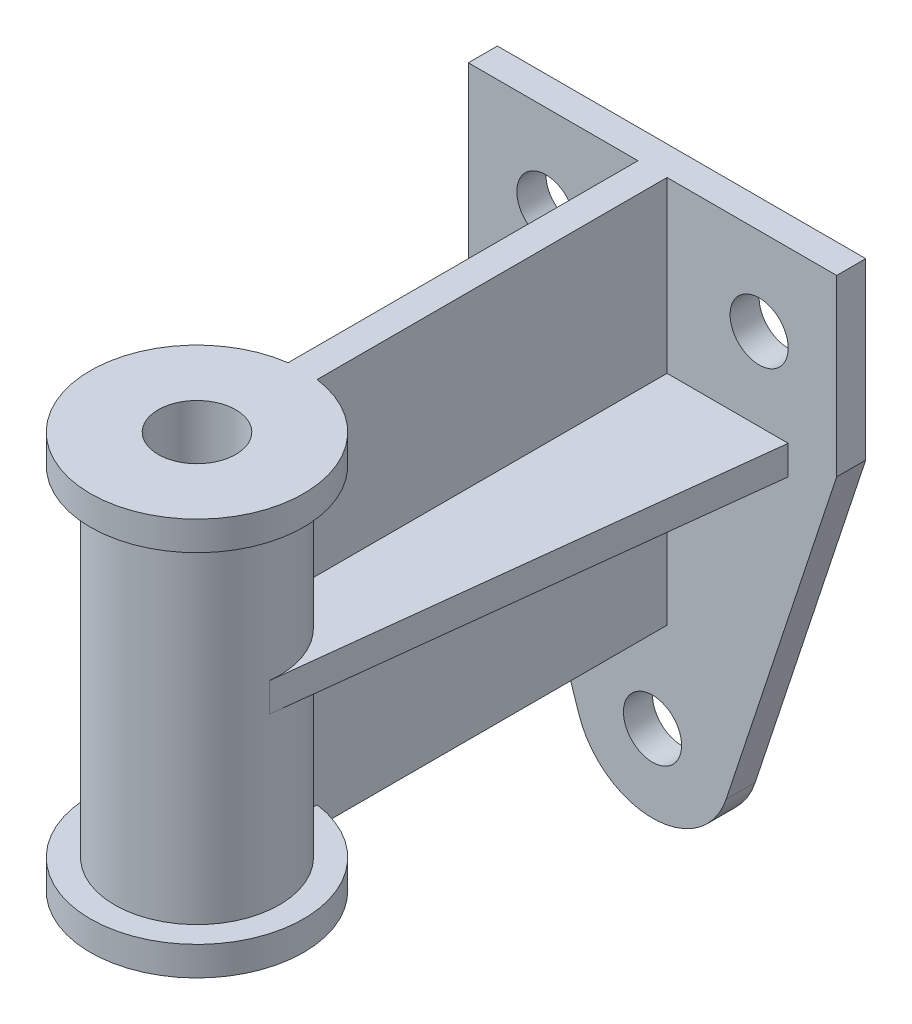
ISO-10303-21;
HEADER;
FILE_DESCRIPTION(('STEP AP214'),'2;1');
FILE_NAME('part.step','',(''),(''),'','','');
FILE_SCHEMA(('AUTOMOTIVE_DESIGN { 1 0 10303 214 1 1 1 1 }'));
ENDSEC;
DATA;
#1=APPLICATION_CONTEXT('core data for automotive mechanical design processes');
#2=APPLICATION_PROTOCOL_DEFINITION('international standard','automotive_design',2000,#1);
#3=PRODUCT_CONTEXT('',#1,'mechanical');
#4=PRODUCT('Part','Part','',(#3));
#5=PRODUCT_RELATED_PRODUCT_CATEGORY('part','',(#4));
#6=PRODUCT_DEFINITION_FORMATION('','',#4);
#7=PRODUCT_DEFINITION_CONTEXT('part definition',#1,'design');
#8=PRODUCT_DEFINITION('design','',#6,#7);
#9=PRODUCT_DEFINITION_SHAPE('','',#8);
#10=(LENGTH_UNIT() NAMED_UNIT(*) SI_UNIT(.MILLI.,.METRE.));
#11=(NAMED_UNIT(*) PLANE_ANGLE_UNIT() SI_UNIT($,.RADIAN.));
#12=(NAMED_UNIT(*) SI_UNIT($,.STERADIAN.) SOLID_ANGLE_UNIT());
#13=UNCERTAINTY_MEASURE_WITH_UNIT(LENGTH_MEASURE(1.E-05),#10,'distance_accuracy_value','');
#14=(GEOMETRIC_REPRESENTATION_CONTEXT(3) GLOBAL_UNCERTAINTY_ASSIGNED_CONTEXT((#13)) GLOBAL_UNIT_ASSIGNED_CONTEXT((#10,
#11,#12)) REPRESENTATION_CONTEXT('',''));
#15=CARTESIAN_POINT('',(0.,0.,0.));
#16=DIRECTION('',(0.,0.,1.));
#17=DIRECTION('',(1.,0.,0.));
#18=AXIS2_PLACEMENT_3D('',#15,#16,#17);
#19=CARTESIAN_POINT('',(0.,0.,6.));
#20=DIRECTION('',(0.,0.,1.));
#21=DIRECTION('',(1.,0.,0.));
#22=AXIS2_PLACEMENT_3D('',#19,#20,#21);
#23=PLANE('',#22);
#24=CARTESIAN_POINT('',(0.,0.,6.));
#25=DIRECTION('',(0.,0.,1.));
#26=DIRECTION('',(1.,0.,0.));
#27=AXIS2_PLACEMENT_3D('',#24,#25,#26);
#28=CIRCLE('',#27,6.);
#29=CARTESIAN_POINT('',(6.,0.,6.));
#30=VERTEX_POINT('',#29);
#31=EDGE_CURVE('E232',#30,#30,#28,.T.);
#32=ORIENTED_EDGE('',*,*,#31,.F.);
#33=EDGE_LOOP('',(#32));
#34=FACE_BOUND('',#33,.T.);
#35=CARTESIAN_POINT('',(-22.,82.,6.));
#36=DIRECTION('',(0.,0.,1.));
#37=DIRECTION('',(1.,0.,0.));
#38=AXIS2_PLACEMENT_3D('',#35,#36,#37);
#39=CIRCLE('',#38,6.);
#40=CARTESIAN_POINT('',(-16.,82.,6.));
#41=VERTEX_POINT('',#40);
#42=EDGE_CURVE('E240',#41,#41,#39,.T.);
#43=ORIENTED_EDGE('',*,*,#42,.F.);
#44=EDGE_LOOP('',(#43));
#45=FACE_BOUND('',#44,.T.);
#46=CARTESIAN_POINT('',(22.,82.,6.));
#47=DIRECTION('',(0.,0.,1.));
#48=DIRECTION('',(1.,0.,0.));
#49=AXIS2_PLACEMENT_3D('',#46,#47,#48);
#50=CIRCLE('',#49,6.);
#51=CARTESIAN_POINT('',(28.,82.,6.));
#52=VERTEX_POINT('',#51);
#53=EDGE_CURVE('E241',#52,#52,#50,.T.);
#54=ORIENTED_EDGE('',*,*,#53,.F.);
#55=EDGE_LOOP('',(#54));
#56=FACE_BOUND('',#55,.T.);
#57=DIRECTION('',(-1.,0.,0.));
#58=VECTOR('',#57,1.);
#59=CARTESIAN_POINT('',(-28.,59.,6.));
#60=LINE('',#59,#58);
#61=CARTESIAN_POINT('',(28.,59.,6.));
#62=VERTEX_POINT('',#61);
#63=CARTESIAN_POINT('',(2.99999999999999,59.,6.));
#64=VERTEX_POINT('',#63);
#65=EDGE_CURVE('E308',#62,#64,#60,.T.);
#66=ORIENTED_EDGE('',*,*,#65,.T.);
#67=DIRECTION('',(0.,1.,0.));
#68=VECTOR('',#67,1.);
#69=CARTESIAN_POINT('',(2.99999999999999,59.,6.));
#70=LINE('',#69,#68);
#71=CARTESIAN_POINT('',(3.,20.,6.));
#72=VERTEX_POINT('',#71);
#73=EDGE_CURVE('E61',#72,#64,#70,.T.);
#74=ORIENTED_EDGE('',*,*,#73,.F.);
#75=DIRECTION('',(1.,0.,0.));
#76=VECTOR('',#75,1.);
#77=CARTESIAN_POINT('',(-3.,20.,6.));
#78=LINE('',#77,#76);
#79=CARTESIAN_POINT('',(-3.,20.,6.));
#80=VERTEX_POINT('',#79);
#81=EDGE_CURVE('E59',#80,#72,#78,.T.);
#82=ORIENTED_EDGE('',*,*,#81,.F.);
#83=DIRECTION('',(0.,-1.,0.));
#84=VECTOR('',#83,1.);
#85=CARTESIAN_POINT('',(-3.00000000000001,59.,6.));
#86=LINE('',#85,#84);
#87=CARTESIAN_POINT('',(-3.00000000000001,59.,6.));
#88=VERTEX_POINT('',#87);
#89=EDGE_CURVE('E247',#88,#80,#86,.T.);
#90=ORIENTED_EDGE('',*,*,#89,.F.);
#91=CARTESIAN_POINT('',(-28.,59.,6.));
#92=VERTEX_POINT('',#91);
#93=EDGE_CURVE('E301',#88,#92,#60,.T.);
#94=ORIENTED_EDGE('',*,*,#93,.T.);
#95=DIRECTION('',(0.,1.,0.));
#96=VECTOR('',#95,1.);
#97=CARTESIAN_POINT('',(-28.,59.,6.));
#98=LINE('',#97,#96);
#99=CARTESIAN_POINT('',(-28.,65.,6.));
#100=VERTEX_POINT('',#99);
#101=EDGE_CURVE('E321',#92,#100,#98,.T.);
#102=ORIENTED_EDGE('',*,*,#101,.T.);
#103=DIRECTION('',(-1.,0.,0.));
#104=VECTOR('',#103,1.);
#105=CARTESIAN_POINT('',(-28.,65.,6.));
#106=LINE('',#105,#104);
#107=CARTESIAN_POINT('',(-3.00000000000001,65.,6.));
#108=VERTEX_POINT('',#107);
#109=EDGE_CURVE('E318',#108,#100,#106,.T.);
#110=ORIENTED_EDGE('',*,*,#109,.F.);
#111=DIRECTION('',(0.,-1.,0.));
#112=VECTOR('',#111,1.);
#113=CARTESIAN_POINT('',(-3.00000000000002,100.,6.));
#114=LINE('',#113,#112);
#115=CARTESIAN_POINT('',(-3.00000000000002,100.,6.));
#116=VERTEX_POINT('',#115);
#117=EDGE_CURVE('E246',#116,#108,#114,.T.);
#118=ORIENTED_EDGE('',*,*,#117,.F.);
#119=DIRECTION('',(-1.,0.,0.));
#120=VECTOR('',#119,1.);
#121=CARTESIAN_POINT('',(-38.,100.,6.));
#122=LINE('',#121,#120);
#123=CARTESIAN_POINT('',(-38.,100.,6.));
#124=VERTEX_POINT('',#123);
#125=EDGE_CURVE('E341',#116,#124,#122,.T.);
#126=ORIENTED_EDGE('',*,*,#125,.T.);
#127=DIRECTION('',(0.,-1.,0.));
#128=VECTOR('',#127,1.);
#129=CARTESIAN_POINT('',(-38.,100.,6.));
#130=LINE('',#129,#128);
#131=CARTESIAN_POINT('',(-38.,64.,6.));
#132=VERTEX_POINT('',#131);
#133=EDGE_CURVE('E334',#124,#132,#130,.T.);
#134=ORIENTED_EDGE('',*,*,#133,.T.);
#135=DIRECTION('',(0.313765855685688,-0.949500388523264,0.));
#136=VECTOR('',#135,1.);
#137=CARTESIAN_POINT('',(-38.,64.,6.));
#138=LINE('',#137,#136);
#139=CARTESIAN_POINT('',(-15.1920062163722,-5.020253690971,6.));
#140=VERTEX_POINT('',#139);
#141=EDGE_CURVE('E338',#132,#140,#138,.T.);
#142=ORIENTED_EDGE('',*,*,#141,.T.);
#143=CARTESIAN_POINT('',(0.,0.,6.));
#144=DIRECTION('',(0.,0.,1.));
#145=DIRECTION('',(1.,0.,0.));
#146=AXIS2_PLACEMENT_3D('',#143,#144,#145);
#147=CIRCLE('',#146,16.);
#148=CARTESIAN_POINT('',(15.1920062163722,-5.020253690971,6.));
#149=VERTEX_POINT('',#148);
#150=EDGE_CURVE('E337',#140,#149,#147,.T.);
#151=ORIENTED_EDGE('',*,*,#150,.T.);
#152=DIRECTION('',(0.313765855685688,0.949500388523264,0.));
#153=VECTOR('',#152,1.);
#154=CARTESIAN_POINT('',(38.,64.,6.));
#155=LINE('',#154,#153);
#156=CARTESIAN_POINT('',(38.,64.,6.));
#157=VERTEX_POINT('',#156);
#158=EDGE_CURVE('E342',#149,#157,#155,.T.);
#159=ORIENTED_EDGE('',*,*,#158,.T.);
#160=DIRECTION('',(0.,1.,0.));
#161=VECTOR('',#160,1.);
#162=CARTESIAN_POINT('',(38.,100.,6.));
#163=LINE('',#162,#161);
#164=CARTESIAN_POINT('',(38.,100.,6.));
#165=VERTEX_POINT('',#164);
#166=EDGE_CURVE('E343',#157,#165,#163,.T.);
#167=ORIENTED_EDGE('',*,*,#166,.T.);
#168=CARTESIAN_POINT('',(2.99999999999998,100.,6.));
#169=VERTEX_POINT('',#168);
#170=EDGE_CURVE('E347',#165,#169,#122,.T.);
#171=ORIENTED_EDGE('',*,*,#170,.T.);
#172=DIRECTION('',(0.,1.,0.));
#173=VECTOR('',#172,1.);
#174=CARTESIAN_POINT('',(2.99999999999998,100.,6.));
#175=LINE('',#174,#173);
#176=CARTESIAN_POINT('',(2.99999999999999,65.,6.));
#177=VERTEX_POINT('',#176);
#178=EDGE_CURVE('E250',#177,#169,#175,.T.);
#179=ORIENTED_EDGE('',*,*,#178,.F.);
#180=CARTESIAN_POINT('',(28.,65.,6.));
#181=VERTEX_POINT('',#180);
#182=EDGE_CURVE('E299',#181,#177,#106,.T.);
#183=ORIENTED_EDGE('',*,*,#182,.F.);
#184=DIRECTION('',(0.,1.,0.));
#185=VECTOR('',#184,1.);
#186=CARTESIAN_POINT('',(28.,59.,5.99999999999999));
#187=LINE('',#186,#185);
#188=EDGE_CURVE('E324',#62,#181,#187,.T.);
#189=ORIENTED_EDGE('',*,*,#188,.F.);
#190=EDGE_LOOP('',(#66,#74,#82,#90,#94,#102,#110,#118,#126,#134,#142,#151,#159,#167,#171,#179,
#183,#189));
#191=FACE_BOUND('',#190,.T.);
#192=ADVANCED_FACE('F43',(#34,#45,#56,#191),#23,.T.);
#193=CARTESIAN_POINT('',(0.,24.,100.));
#194=DIRECTION('',(0.,1.,0.));
#195=DIRECTION('',(-1.,0.,0.));
#196=AXIS2_PLACEMENT_3D('',#193,#194,#195);
#197=CYLINDRICAL_SURFACE('',#196,17.);
#198=DIRECTION('',(0.,1.,0.));
#199=VECTOR('',#198,1.);
#200=CARTESIAN_POINT('',(3.,24.,83.2667994693185));
#201=LINE('',#200,#199);
#202=CARTESIAN_POINT('',(3.,24.,83.2667994693185));
#203=VERTEX_POINT('',#202);
#204=CARTESIAN_POINT('',(2.99999999999999,59.,83.2667994693185));
#205=VERTEX_POINT('',#204);
#206=EDGE_CURVE('E432',#203,#205,#201,.T.);
#207=ORIENTED_EDGE('',*,*,#206,.T.);
#208=CARTESIAN_POINT('',(0.,59.,100.));
#209=DIRECTION('',(0.,-1.,0.));
#210=DIRECTION('',(0.,0.,1.));
#211=AXIS2_PLACEMENT_3D('',#208,#209,#210);
#212=CIRCLE('',#211,17.);
#213=CARTESIAN_POINT('',(16.887127655556,59.,101.955740152719));
#214=VERTEX_POINT('',#213);
#215=EDGE_CURVE('E297',#205,#214,#212,.T.);
#216=ORIENTED_EDGE('',*,*,#215,.T.);
#217=DIRECTION('',(0.,1.,0.));
#218=VECTOR('',#217,1.);
#219=CARTESIAN_POINT('',(16.887127655556,59.,101.955740152719));
#220=LINE('',#219,#218);
#221=CARTESIAN_POINT('',(16.887127655556,65.,101.955740152719));
#222=VERTEX_POINT('',#221);
#223=EDGE_CURVE('E327',#214,#222,#220,.T.);
#224=ORIENTED_EDGE('',*,*,#223,.T.);
#225=CARTESIAN_POINT('',(0.,65.,100.));
#226=DIRECTION('',(0.,-1.,0.));
#227=DIRECTION('',(0.,0.,1.));
#228=AXIS2_PLACEMENT_3D('',#225,#226,#227);
#229=CIRCLE('',#228,17.);
#230=CARTESIAN_POINT('',(2.99999999999999,65.,83.2667994693185));
#231=VERTEX_POINT('',#230);
#232=EDGE_CURVE('E313',#231,#222,#229,.T.);
#233=ORIENTED_EDGE('',*,*,#232,.F.);
#234=DIRECTION('',(0.,1.,0.));
#235=VECTOR('',#234,1.);
#236=CARTESIAN_POINT('',(2.99999999999999,24.,83.2667994693185));
#237=LINE('',#236,#235);
#238=CARTESIAN_POINT('',(3.00000000000001,94.,83.2667994693185));
#239=VERTEX_POINT('',#238);
#240=EDGE_CURVE('E229',#231,#239,#237,.T.);
#241=ORIENTED_EDGE('',*,*,#240,.T.);
#242=CARTESIAN_POINT('',(0.,94.,100.));
#243=DIRECTION('',(0.,-1.,0.));
#244=DIRECTION('',(1.,0.,0.));
#245=AXIS2_PLACEMENT_3D('',#242,#243,#244);
#246=CIRCLE('',#245,17.);
#247=CARTESIAN_POINT('',(-2.99999999999999,94.,83.2667994693185));
#248=VERTEX_POINT('',#247);
#249=EDGE_CURVE('E284',#239,#248,#246,.T.);
#250=ORIENTED_EDGE('',*,*,#249,.T.);
#251=DIRECTION('',(0.,1.,0.));
#252=VECTOR('',#251,1.);
#253=CARTESIAN_POINT('',(-3.,24.,83.2667994693185));
#254=LINE('',#253,#252);
#255=CARTESIAN_POINT('',(-3.00000000000001,65.,83.2667994693185));
#256=VERTEX_POINT('',#255);
#257=EDGE_CURVE('E261',#248,#256,#254,.F.);
#258=ORIENTED_EDGE('',*,*,#257,.T.);
#259=CARTESIAN_POINT('',(-16.887127655556,65.,101.955740152719));
#260=VERTEX_POINT('',#259);
#261=EDGE_CURVE('E315',#260,#256,#229,.T.);
#262=ORIENTED_EDGE('',*,*,#261,.F.);
#263=DIRECTION('',(0.,1.,0.));
#264=VECTOR('',#263,1.);
#265=CARTESIAN_POINT('',(-16.887127655556,59.,101.955740152719));
#266=LINE('',#265,#264);
#267=CARTESIAN_POINT('',(-16.887127655556,59.,101.955740152719));
#268=VERTEX_POINT('',#267);
#269=EDGE_CURVE('E306',#268,#260,#266,.T.);
#270=ORIENTED_EDGE('',*,*,#269,.F.);
#271=CARTESIAN_POINT('',(-3.00000000000001,59.,83.2667994693185));
#272=VERTEX_POINT('',#271);
#273=EDGE_CURVE('E209',#268,#272,#212,.T.);
#274=ORIENTED_EDGE('',*,*,#273,.T.);
#275=DIRECTION('',(0.,1.,0.));
#276=VECTOR('',#275,1.);
#277=CARTESIAN_POINT('',(-3.,24.,83.2667994693185));
#278=LINE('',#277,#276);
#279=CARTESIAN_POINT('',(-3.,24.,83.2667994693185));
#280=VERTEX_POINT('',#279);
#281=EDGE_CURVE('E210',#272,#280,#278,.F.);
#282=ORIENTED_EDGE('',*,*,#281,.T.);
#283=CARTESIAN_POINT('',(0.,24.,100.));
#284=DIRECTION('',(0.,-1.,0.));
#285=DIRECTION('',(1.,0.,0.));
#286=AXIS2_PLACEMENT_3D('',#283,#284,#285);
#287=CIRCLE('',#286,17.);
#288=EDGE_CURVE('E192',#203,#280,#287,.T.);
#289=ORIENTED_EDGE('',*,*,#288,.F.);
#290=EDGE_LOOP('',(#207,#216,#224,#233,#241,#250,#258,#262,#270,#274,#282,#289));
#291=FACE_BOUND('',#290,.T.);
#292=ADVANCED_FACE('F208',(#291),#197,.T.);
#293=CARTESIAN_POINT('',(0.,59.,100.));
#294=DIRECTION('',(0.,1.,0.));
#295=DIRECTION('',(0.,0.,1.));
#296=AXIS2_PLACEMENT_3D('',#293,#294,#295);
#297=PLANE('',#296);
#298=DIRECTION('',(0.,0.,-1.));
#299=VECTOR('',#298,1.);
#300=CARTESIAN_POINT('',(2.99999999999999,59.,122.002));
#301=LINE('',#300,#299);
#302=EDGE_CURVE('E421',#205,#64,#301,.T.);
#303=ORIENTED_EDGE('',*,*,#302,.T.);
#304=ORIENTED_EDGE('',*,*,#65,.F.);
#305=DIRECTION('',(0.115043538395224,0.,-0.993360450326822));
#306=VECTOR('',#305,1.);
#307=CARTESIAN_POINT('',(28.,59.,5.99999999999999));
#308=LINE('',#307,#306);
#309=EDGE_CURVE('E305',#214,#62,#308,.T.);
#310=ORIENTED_EDGE('',*,*,#309,.F.);
#311=ORIENTED_EDGE('',*,*,#215,.F.);
#312=EDGE_LOOP('',(#303,#304,#310,#311));
#313=FACE_BOUND('',#312,.T.);
#314=ADVANCED_FACE('F480',(#313),#297,.F.);
#315=DIRECTION('',(0.,0.,-1.));
#316=VECTOR('',#315,1.);
#317=CARTESIAN_POINT('',(-3.00000000000001,59.,122.002));
#318=LINE('',#317,#316);
#319=EDGE_CURVE('E426',#272,#88,#318,.T.);
#320=ORIENTED_EDGE('',*,*,#319,.F.);
#321=ORIENTED_EDGE('',*,*,#273,.F.);
#322=DIRECTION('',(0.115043538395223,0.,0.993360450326822));
#323=VECTOR('',#322,1.);
#324=CARTESIAN_POINT('',(-28.,59.,6.));
#325=LINE('',#324,#323);
#326=EDGE_CURVE('E298',#92,#268,#325,.T.);
#327=ORIENTED_EDGE('',*,*,#326,.F.);
#328=ORIENTED_EDGE('',*,*,#93,.F.);
#329=EDGE_LOOP('',(#320,#321,#327,#328));
#330=FACE_BOUND('',#329,.T.);
#331=ADVANCED_FACE('F441',(#330),#297,.F.);
#332=CARTESIAN_POINT('',(0.,18.,100.));
#333=DIRECTION('',(0.,1.,0.));
#334=DIRECTION('',(-1.,0.,0.));
#335=AXIS2_PLACEMENT_3D('',#332,#333,#334);
#336=CYLINDRICAL_SURFACE('',#335,22.);
#337=CARTESIAN_POINT('',(0.,18.,100.));
#338=DIRECTION('',(0.,-1.,0.));
#339=DIRECTION('',(1.,0.,0.));
#340=AXIS2_PLACEMENT_3D('',#337,#338,#339);
#341=CIRCLE('',#340,22.);
#342=CARTESIAN_POINT('',(22.,18.,100.));
#343=VERTEX_POINT('',#342);
#344=EDGE_CURVE('E201',#343,#343,#341,.T.);
#345=ORIENTED_EDGE('',*,*,#344,.F.);
#346=EDGE_LOOP('',(#345));
#347=FACE_BOUND('',#346,.T.);
#348=DIRECTION('',(0.,1.,0.));
#349=VECTOR('',#348,1.);
#350=CARTESIAN_POINT('',(3.,18.,78.2055052822966));
#351=LINE('',#350,#349);
#352=CARTESIAN_POINT('',(3.,20.,78.2055052822966));
#353=VERTEX_POINT('',#352);
#354=CARTESIAN_POINT('',(3.,24.,78.2055052822966));
#355=VERTEX_POINT('',#354);
#356=EDGE_CURVE('E228',#353,#355,#351,.T.);
#357=ORIENTED_EDGE('',*,*,#356,.T.);
#358=CARTESIAN_POINT('',(0.,24.,100.));
#359=DIRECTION('',(0.,-1.,0.));
#360=DIRECTION('',(1.,0.,0.));
#361=AXIS2_PLACEMENT_3D('',#358,#359,#360);
#362=CIRCLE('',#361,22.);
#363=CARTESIAN_POINT('',(-3.,24.,78.2055052822966));
#364=VERTEX_POINT('',#363);
#365=EDGE_CURVE('E281',#355,#364,#362,.T.);
#366=ORIENTED_EDGE('',*,*,#365,.T.);
#367=DIRECTION('',(0.,1.,0.));
#368=VECTOR('',#367,1.);
#369=CARTESIAN_POINT('',(-3.,18.,78.2055052822966));
#370=LINE('',#369,#368);
#371=CARTESIAN_POINT('',(-3.,20.,78.2055052822966));
#372=VERTEX_POINT('',#371);
#373=EDGE_CURVE('E217',#364,#372,#370,.F.);
#374=ORIENTED_EDGE('',*,*,#373,.T.);
#375=CARTESIAN_POINT('',(0.,20.,100.));
#376=DIRECTION('',(0.,1.,0.));
#377=DIRECTION('',(-1.,0.,0.));
#378=AXIS2_PLACEMENT_3D('',#375,#376,#377);
#379=CIRCLE('',#378,22.);
#380=EDGE_CURVE('E213',#372,#353,#379,.F.);
#381=ORIENTED_EDGE('',*,*,#380,.T.);
#382=EDGE_LOOP('',(#357,#366,#374,#381));
#383=FACE_BOUND('',#382,.T.);
#384=ADVANCED_FACE('F644',(#347,#383),#336,.T.);
#385=CARTESIAN_POINT('',(0.,24.,100.));
#386=DIRECTION('',(0.,-1.,0.));
#387=DIRECTION('',(1.,0.,0.));
#388=AXIS2_PLACEMENT_3D('',#385,#386,#387);
#389=PLANE('',#388);
#390=DIRECTION('',(0.,0.,1.));
#391=VECTOR('',#390,1.);
#392=CARTESIAN_POINT('',(3.,24.,122.002));
#393=LINE('',#392,#391);
#394=EDGE_CURVE('E200',#355,#203,#393,.T.);
#395=ORIENTED_EDGE('',*,*,#394,.T.);
#396=ORIENTED_EDGE('',*,*,#288,.T.);
#397=DIRECTION('',(0.,0.,-1.));
#398=VECTOR('',#397,1.);
#399=CARTESIAN_POINT('',(-3.,24.,122.002));
#400=LINE('',#399,#398);
#401=EDGE_CURVE('E198',#280,#364,#400,.T.);
#402=ORIENTED_EDGE('',*,*,#401,.T.);
#403=ORIENTED_EDGE('',*,*,#365,.F.);
#404=EDGE_LOOP('',(#395,#396,#402,#403));
#405=FACE_BOUND('',#404,.T.);
#406=ADVANCED_FACE('F193',(#405),#389,.F.);
#407=CARTESIAN_POINT('',(0.,65.,100.));
#408=DIRECTION('',(0.,1.,0.));
#409=DIRECTION('',(0.,0.,1.));
#410=AXIS2_PLACEMENT_3D('',#407,#408,#409);
#411=PLANE('',#410);
#412=ORIENTED_EDGE('',*,*,#182,.T.);
#413=DIRECTION('',(0.,0.,-1.));
#414=VECTOR('',#413,1.);
#415=CARTESIAN_POINT('',(2.99999999999999,65.,122.002));
#416=LINE('',#415,#414);
#417=EDGE_CURVE('E275',#231,#177,#416,.T.);
#418=ORIENTED_EDGE('',*,*,#417,.F.);
#419=ORIENTED_EDGE('',*,*,#232,.T.);
#420=DIRECTION('',(0.115043538395224,0.,-0.993360450326822));
#421=VECTOR('',#420,1.);
#422=CARTESIAN_POINT('',(28.,65.,5.99999999999999));
#423=LINE('',#422,#421);
#424=EDGE_CURVE('E312',#222,#181,#423,.T.);
#425=ORIENTED_EDGE('',*,*,#424,.T.);
#426=EDGE_LOOP('',(#412,#418,#419,#425));
#427=FACE_BOUND('',#426,.T.);
#428=ADVANCED_FACE('F409',(#427),#411,.T.);
#429=ORIENTED_EDGE('',*,*,#261,.T.);
#430=DIRECTION('',(0.,0.,-1.));
#431=VECTOR('',#430,1.);
#432=CARTESIAN_POINT('',(-3.00000000000001,65.,122.002));
#433=LINE('',#432,#431);
#434=EDGE_CURVE('E258',#256,#108,#433,.T.);
#435=ORIENTED_EDGE('',*,*,#434,.T.);
#436=ORIENTED_EDGE('',*,*,#109,.T.);
#437=DIRECTION('',(0.115043538395223,0.,0.993360450326822));
#438=VECTOR('',#437,1.);
#439=CARTESIAN_POINT('',(-28.,65.,6.));
#440=LINE('',#439,#438);
#441=EDGE_CURVE('E288',#100,#260,#440,.T.);
#442=ORIENTED_EDGE('',*,*,#441,.T.);
#443=EDGE_LOOP('',(#429,#435,#436,#442));
#444=FACE_BOUND('',#443,.T.);
#445=ADVANCED_FACE('F452',(#444),#411,.T.);
#446=CARTESIAN_POINT('',(0.,94.,100.));
#447=DIRECTION('',(0.,1.,0.));
#448=DIRECTION('',(-1.,0.,0.));
#449=AXIS2_PLACEMENT_3D('',#446,#447,#448);
#450=CYLINDRICAL_SURFACE('',#449,22.);
#451=CARTESIAN_POINT('',(0.,94.,100.));
#452=DIRECTION('',(0.,1.,0.));
#453=DIRECTION('',(-1.,0.,0.));
#454=AXIS2_PLACEMENT_3D('',#451,#452,#453);
#455=CIRCLE('',#454,22.);
#456=CARTESIAN_POINT('',(-3.00000000000002,94.,78.2055052822966));
#457=VERTEX_POINT('',#456);
#458=CARTESIAN_POINT('',(2.99999999999998,94.,78.2055052822966));
#459=VERTEX_POINT('',#458);
#460=EDGE_CURVE('E289',#457,#459,#455,.T.);
#461=ORIENTED_EDGE('',*,*,#460,.T.);
#462=DIRECTION('',(0.,1.,0.));
#463=VECTOR('',#462,1.);
#464=CARTESIAN_POINT('',(2.99999999999998,94.,78.2055052822966));
#465=LINE('',#464,#463);
#466=CARTESIAN_POINT('',(2.99999999999998,100.,78.2055052822966));
#467=VERTEX_POINT('',#466);
#468=EDGE_CURVE('E255',#467,#459,#465,.F.);
#469=ORIENTED_EDGE('',*,*,#468,.F.);
#470=CARTESIAN_POINT('',(0.,100.,100.));
#471=DIRECTION('',(0.,1.,0.));
#472=DIRECTION('',(-1.,0.,0.));
#473=AXIS2_PLACEMENT_3D('',#470,#471,#472);
#474=CIRCLE('',#473,22.);
#475=CARTESIAN_POINT('',(-3.00000000000002,100.,78.2055052822966));
#476=VERTEX_POINT('',#475);
#477=EDGE_CURVE('E205',#476,#467,#474,.T.);
#478=ORIENTED_EDGE('',*,*,#477,.F.);
#479=DIRECTION('',(0.,1.,0.));
#480=VECTOR('',#479,1.);
#481=CARTESIAN_POINT('',(-3.00000000000002,94.,78.2055052822966));
#482=LINE('',#481,#480);
#483=EDGE_CURVE('E260',#457,#476,#482,.T.);
#484=ORIENTED_EDGE('',*,*,#483,.F.);
#485=EDGE_LOOP('',(#461,#469,#478,#484));
#486=FACE_BOUND('',#485,.T.);
#487=ADVANCED_FACE('F458',(#486),#450,.T.);
#488=CARTESIAN_POINT('',(0.,94.,100.));
#489=DIRECTION('',(0.,1.,0.));
#490=DIRECTION('',(-1.,0.,0.));
#491=AXIS2_PLACEMENT_3D('',#488,#489,#490);
#492=PLANE('',#491);
#493=DIRECTION('',(0.,0.,-1.));
#494=VECTOR('',#493,1.);
#495=CARTESIAN_POINT('',(2.99999999999998,94.,122.002));
#496=LINE('',#495,#494);
#497=EDGE_CURVE('E262',#239,#459,#496,.T.);
#498=ORIENTED_EDGE('',*,*,#497,.T.);
#499=ORIENTED_EDGE('',*,*,#460,.F.);
#500=DIRECTION('',(0.,0.,1.));
#501=VECTOR('',#500,1.);
#502=CARTESIAN_POINT('',(-3.00000000000002,94.,122.002));
#503=LINE('',#502,#501);
#504=EDGE_CURVE('E257',#457,#248,#503,.T.);
#505=ORIENTED_EDGE('',*,*,#504,.T.);
#506=ORIENTED_EDGE('',*,*,#249,.F.);
#507=EDGE_LOOP('',(#498,#499,#505,#506));
#508=FACE_BOUND('',#507,.T.);
#509=ADVANCED_FACE('F457',(#508),#492,.F.);
#510=CARTESIAN_POINT('',(-38.,100.,6.));
#511=DIRECTION('',(1.,0.,0.));
#512=DIRECTION('',(0.,1.,0.));
#513=AXIS2_PLACEMENT_3D('',#510,#511,#512);
#514=PLANE('',#513);
#515=DIRECTION('',(0.,-1.,0.));
#516=VECTOR('',#515,1.);
#517=CARTESIAN_POINT('',(-38.,100.,0.));
#518=LINE('',#517,#516);
#519=CARTESIAN_POINT('',(-38.,100.,0.));
#520=VERTEX_POINT('',#519);
#521=CARTESIAN_POINT('',(-38.,64.,0.));
#522=VERTEX_POINT('',#521);
#523=EDGE_CURVE('E322',#520,#522,#518,.T.);
#524=ORIENTED_EDGE('',*,*,#523,.T.);
#525=DIRECTION('',(0.,0.,-1.));
#526=VECTOR('',#525,1.);
#527=CARTESIAN_POINT('',(-38.,64.,6.));
#528=LINE('',#527,#526);
#529=EDGE_CURVE('E11',#132,#522,#528,.T.);
#530=ORIENTED_EDGE('',*,*,#529,.F.);
#531=ORIENTED_EDGE('',*,*,#133,.F.);
#532=DIRECTION('',(0.,0.,-1.));
#533=VECTOR('',#532,1.);
#534=CARTESIAN_POINT('',(-38.,100.,6.));
#535=LINE('',#534,#533);
#536=EDGE_CURVE('E349',#124,#520,#535,.T.);
#537=ORIENTED_EDGE('',*,*,#536,.T.);
#538=EDGE_LOOP('',(#524,#530,#531,#537));
#539=FACE_BOUND('',#538,.T.);
#540=ADVANCED_FACE('F44',(#539),#514,.F.);
#541=CARTESIAN_POINT('',(-38.,64.,6.));
#542=DIRECTION('',(0.949500388523263,0.313765855685687,0.));
#543=DIRECTION('',(-0.313765855685688,0.949500388523264,0.));
#544=AXIS2_PLACEMENT_3D('',#541,#542,#543);
#545=PLANE('',#544);
#546=DIRECTION('',(0.313765855685688,-0.949500388523264,0.));
#547=VECTOR('',#546,1.);
#548=CARTESIAN_POINT('',(-38.,64.,0.));
#549=LINE('',#548,#547);
#550=CARTESIAN_POINT('',(-15.1920062163722,-5.020253690971,0.));
#551=VERTEX_POINT('',#550);
#552=EDGE_CURVE('E355',#522,#551,#549,.T.);
#553=ORIENTED_EDGE('',*,*,#552,.T.);
#554=DIRECTION('',(0.,0.,-1.));
#555=VECTOR('',#554,1.);
#556=CARTESIAN_POINT('',(-15.1920062163722,-5.020253690971,6.));
#557=LINE('',#556,#555);
#558=EDGE_CURVE('E51',#140,#551,#557,.T.);
#559=ORIENTED_EDGE('',*,*,#558,.F.);
#560=ORIENTED_EDGE('',*,*,#141,.F.);
#561=ORIENTED_EDGE('',*,*,#529,.T.);
#562=EDGE_LOOP('',(#553,#559,#560,#561));
#563=FACE_BOUND('',#562,.T.);
#564=ADVANCED_FACE('F400',(#563),#545,.F.);
#565=CARTESIAN_POINT('',(0.,0.,6.));
#566=DIRECTION('',(0.,0.,-1.));
#567=DIRECTION('',(-1.,0.,0.));
#568=AXIS2_PLACEMENT_3D('',#565,#566,#567);
#569=CYLINDRICAL_SURFACE('',#568,16.);
#570=CARTESIAN_POINT('',(0.,0.,0.));
#571=DIRECTION('',(0.,0.,1.));
#572=DIRECTION('',(1.,0.,0.));
#573=AXIS2_PLACEMENT_3D('',#570,#571,#572);
#574=CIRCLE('',#573,16.);
#575=CARTESIAN_POINT('',(15.1920062163722,-5.020253690971,0.));
#576=VERTEX_POINT('',#575);
#577=EDGE_CURVE('E352',#551,#576,#574,.T.);
#578=ORIENTED_EDGE('',*,*,#577,.T.);
#579=DIRECTION('',(0.,0.,-1.));
#580=VECTOR('',#579,1.);
#581=CARTESIAN_POINT('',(15.1920062163722,-5.020253690971,6.));
#582=LINE('',#581,#580);
#583=EDGE_CURVE('E369',#149,#576,#582,.T.);
#584=ORIENTED_EDGE('',*,*,#583,.F.);
#585=ORIENTED_EDGE('',*,*,#150,.F.);
#586=ORIENTED_EDGE('',*,*,#558,.T.);
#587=EDGE_LOOP('',(#578,#584,#585,#586));
#588=FACE_BOUND('',#587,.T.);
#589=ADVANCED_FACE('F376',(#588),#569,.T.);
#590=CARTESIAN_POINT('',(38.,64.,6.));
#591=DIRECTION('',(-0.949500388523263,0.313765855685687,0.));
#592=DIRECTION('',(-0.313765855685688,-0.949500388523264,0.));
#593=AXIS2_PLACEMENT_3D('',#590,#591,#592);
#594=PLANE('',#593);
#595=DIRECTION('',(0.313765855685688,0.949500388523264,0.));
#596=VECTOR('',#595,1.);
#597=CARTESIAN_POINT('',(38.,64.,0.));
#598=LINE('',#597,#596);
#599=CARTESIAN_POINT('',(38.,64.,0.));
#600=VERTEX_POINT('',#599);
#601=EDGE_CURVE('E357',#576,#600,#598,.T.);
#602=ORIENTED_EDGE('',*,*,#601,.T.);
#603=DIRECTION('',(0.,0.,-1.));
#604=VECTOR('',#603,1.);
#605=CARTESIAN_POINT('',(38.,64.,6.));
#606=LINE('',#605,#604);
#607=EDGE_CURVE('E368',#157,#600,#606,.T.);
#608=ORIENTED_EDGE('',*,*,#607,.F.);
#609=ORIENTED_EDGE('',*,*,#158,.F.);
#610=ORIENTED_EDGE('',*,*,#583,.T.);
#611=EDGE_LOOP('',(#602,#608,#609,#610));
#612=FACE_BOUND('',#611,.T.);
#613=ADVANCED_FACE('F390',(#612),#594,.F.);
#614=CARTESIAN_POINT('',(38.,100.,6.));
#615=DIRECTION('',(-1.,0.,0.));
#616=DIRECTION('',(0.,-1.,0.));
#617=AXIS2_PLACEMENT_3D('',#614,#615,#616);
#618=PLANE('',#617);
#619=DIRECTION('',(0.,1.,0.));
#620=VECTOR('',#619,1.);
#621=CARTESIAN_POINT('',(38.,100.,0.));
#622=LINE('',#621,#620);
#623=CARTESIAN_POINT('',(38.,100.,0.));
#624=VERTEX_POINT('',#623);
#625=EDGE_CURVE('E358',#600,#624,#622,.T.);
#626=ORIENTED_EDGE('',*,*,#625,.T.);
#627=DIRECTION('',(0.,0.,-1.));
#628=VECTOR('',#627,1.);
#629=CARTESIAN_POINT('',(38.,100.,6.));
#630=LINE('',#629,#628);
#631=EDGE_CURVE('E361',#165,#624,#630,.T.);
#632=ORIENTED_EDGE('',*,*,#631,.F.);
#633=ORIENTED_EDGE('',*,*,#166,.F.);
#634=ORIENTED_EDGE('',*,*,#607,.T.);
#635=EDGE_LOOP('',(#626,#632,#633,#634));
#636=FACE_BOUND('',#635,.T.);
#637=ADVANCED_FACE('F393',(#636),#618,.F.);
#638=CARTESIAN_POINT('',(-38.,100.,6.));
#639=DIRECTION('',(0.,-1.,0.));
#640=DIRECTION('',(1.,0.,0.));
#641=AXIS2_PLACEMENT_3D('',#638,#639,#640);
#642=PLANE('',#641);
#643=DIRECTION('',(-1.,0.,0.));
#644=VECTOR('',#643,1.);
#645=CARTESIAN_POINT('',(-38.,100.,0.));
#646=LINE('',#645,#644);
#647=EDGE_CURVE('E340',#624,#520,#646,.T.);
#648=ORIENTED_EDGE('',*,*,#647,.T.);
#649=ORIENTED_EDGE('',*,*,#536,.F.);
#650=ORIENTED_EDGE('',*,*,#125,.F.);
#651=DIRECTION('',(0.,0.,-1.));
#652=VECTOR('',#651,1.);
#653=CARTESIAN_POINT('',(-3.00000000000002,100.,122.002));
#654=LINE('',#653,#652);
#655=EDGE_CURVE('E253',#476,#116,#654,.T.);
#656=ORIENTED_EDGE('',*,*,#655,.F.);
#657=ORIENTED_EDGE('',*,*,#477,.T.);
#658=DIRECTION('',(0.,0.,-1.));
#659=VECTOR('',#658,1.);
#660=CARTESIAN_POINT('',(2.99999999999998,100.,122.002));
#661=LINE('',#660,#659);
#662=EDGE_CURVE('E269',#467,#169,#661,.T.);
#663=ORIENTED_EDGE('',*,*,#662,.T.);
#664=ORIENTED_EDGE('',*,*,#170,.F.);
#665=ORIENTED_EDGE('',*,*,#631,.T.);
#666=EDGE_LOOP('',(#648,#649,#650,#656,#657,#663,#664,#665));
#667=FACE_BOUND('',#666,.T.);
#668=CARTESIAN_POINT('',(0.,100.,100.));
#669=DIRECTION('',(0.,1.,0.));
#670=DIRECTION('',(-1.,0.,0.));
#671=AXIS2_PLACEMENT_3D('',#668,#669,#670);
#672=CIRCLE('',#671,8.);
#673=CARTESIAN_POINT('',(-8.00000000000002,100.,100.));
#674=VERTEX_POINT('',#673);
#675=EDGE_CURVE('E251',#674,#674,#672,.T.);
#676=ORIENTED_EDGE('',*,*,#675,.F.);
#677=EDGE_LOOP('',(#676));
#678=FACE_BOUND('',#677,.T.);
#679=ADVANCED_FACE('F402',(#667,#678),#642,.F.);
#680=CARTESIAN_POINT('',(0.,0.,0.));
#681=DIRECTION('',(0.,0.,1.));
#682=DIRECTION('',(1.,0.,0.));
#683=AXIS2_PLACEMENT_3D('',#680,#681,#682);
#684=PLANE('',#683);
#685=CARTESIAN_POINT('',(0.,0.,0.));
#686=DIRECTION('',(0.,0.,1.));
#687=DIRECTION('',(1.,0.,0.));
#688=AXIS2_PLACEMENT_3D('',#685,#686,#687);
#689=CIRCLE('',#688,6.);
#690=CARTESIAN_POINT('',(6.,0.,0.));
#691=VERTEX_POINT('',#690);
#692=EDGE_CURVE('E230',#691,#691,#689,.T.);
#693=ORIENTED_EDGE('',*,*,#692,.T.);
#694=EDGE_LOOP('',(#693));
#695=FACE_BOUND('',#694,.T.);
#696=CARTESIAN_POINT('',(-22.,82.,0.));
#697=DIRECTION('',(0.,0.,1.));
#698=DIRECTION('',(1.,0.,0.));
#699=AXIS2_PLACEMENT_3D('',#696,#697,#698);
#700=CIRCLE('',#699,6.);
#701=CARTESIAN_POINT('',(-16.,82.,0.));
#702=VERTEX_POINT('',#701);
#703=EDGE_CURVE('E234',#702,#702,#700,.T.);
#704=ORIENTED_EDGE('',*,*,#703,.T.);
#705=EDGE_LOOP('',(#704));
#706=FACE_BOUND('',#705,.T.);
#707=CARTESIAN_POINT('',(22.,82.,0.));
#708=DIRECTION('',(0.,0.,1.));
#709=DIRECTION('',(1.,0.,0.));
#710=AXIS2_PLACEMENT_3D('',#707,#708,#709);
#711=CIRCLE('',#710,6.);
#712=CARTESIAN_POINT('',(28.,82.,0.));
#713=VERTEX_POINT('',#712);
#714=EDGE_CURVE('E238',#713,#713,#711,.T.);
#715=ORIENTED_EDGE('',*,*,#714,.T.);
#716=EDGE_LOOP('',(#715));
#717=FACE_BOUND('',#716,.T.);
#718=ORIENTED_EDGE('',*,*,#523,.F.);
#719=ORIENTED_EDGE('',*,*,#647,.F.);
#720=ORIENTED_EDGE('',*,*,#625,.F.);
#721=ORIENTED_EDGE('',*,*,#601,.F.);
#722=ORIENTED_EDGE('',*,*,#577,.F.);
#723=ORIENTED_EDGE('',*,*,#552,.F.);
#724=EDGE_LOOP('',(#718,#719,#720,#721,#722,#723));
#725=FACE_BOUND('',#724,.T.);
#726=ADVANCED_FACE('F385',(#695,#706,#717,#725),#684,.F.);
#727=CARTESIAN_POINT('',(-28.,59.,6.));
#728=DIRECTION('',(-0.993360450326822,0.,0.115043538395223));
#729=DIRECTION('',(0.115043538395223,0.,0.993360450326822));
#730=AXIS2_PLACEMENT_3D('',#727,#728,#729);
#731=PLANE('',#730);
#732=ORIENTED_EDGE('',*,*,#441,.F.);
#733=ORIENTED_EDGE('',*,*,#101,.F.);
#734=ORIENTED_EDGE('',*,*,#326,.T.);
#735=ORIENTED_EDGE('',*,*,#269,.T.);
#736=EDGE_LOOP('',(#732,#733,#734,#735));
#737=FACE_BOUND('',#736,.T.);
#738=ADVANCED_FACE('F450',(#737),#731,.T.);
#739=CARTESIAN_POINT('',(28.,59.,5.99999999999999));
#740=DIRECTION('',(0.993360450326822,0.,0.115043538395224));
#741=DIRECTION('',(0.115043538395224,0.,-0.993360450326822));
#742=AXIS2_PLACEMENT_3D('',#739,#740,#741);
#743=PLANE('',#742);
#744=ORIENTED_EDGE('',*,*,#424,.F.);
#745=ORIENTED_EDGE('',*,*,#223,.F.);
#746=ORIENTED_EDGE('',*,*,#309,.T.);
#747=ORIENTED_EDGE('',*,*,#188,.T.);
#748=EDGE_LOOP('',(#744,#745,#746,#747));
#749=FACE_BOUND('',#748,.T.);
#750=ADVANCED_FACE('F411',(#749),#743,.T.);
#751=CARTESIAN_POINT('',(0.,18.,100.));
#752=DIRECTION('',(0.,-1.,0.));
#753=DIRECTION('',(1.,0.,0.));
#754=AXIS2_PLACEMENT_3D('',#751,#752,#753);
#755=PLANE('',#754);
#756=CARTESIAN_POINT('',(0.,18.,100.));
#757=DIRECTION('',(0.,-1.,0.));
#758=DIRECTION('',(1.,0.,0.));
#759=AXIS2_PLACEMENT_3D('',#756,#757,#758);
#760=CIRCLE('',#759,8.);
#761=CARTESIAN_POINT('',(-8.00000000000003,18.,100.));
#762=VERTEX_POINT('',#761);
#763=EDGE_CURVE('E278',#762,#762,#760,.T.);
#764=ORIENTED_EDGE('',*,*,#763,.F.);
#765=EDGE_LOOP('',(#764));
#766=FACE_BOUND('',#765,.T.);
#767=ORIENTED_EDGE('',*,*,#344,.T.);
#768=EDGE_LOOP('',(#767));
#769=FACE_BOUND('',#768,.T.);
#770=ADVANCED_FACE('F550',(#766,#769),#755,.T.);
#771=CARTESIAN_POINT('',(0.,-16.,100.));
#772=DIRECTION('',(0.,1.,0.));
#773=DIRECTION('',(-1.,0.,0.));
#774=AXIS2_PLACEMENT_3D('',#771,#772,#773);
#775=CYLINDRICAL_SURFACE('',#774,8.);
#776=CARTESIAN_POINT('',(-8.00000000000003,18.,100.));
#777=CARTESIAN_POINT('',(-8.00000000000003,18.8541666666667,100.));
#778=CARTESIAN_POINT('',(-8.00000000000003,19.7083333333333,100.));
#779=CARTESIAN_POINT('',(-8.00000000000003,21.4166666666667,100.));
#780=CARTESIAN_POINT('',(-8.00000000000003,22.2708333333333,100.));
#781=CARTESIAN_POINT('',(-8.00000000000003,23.9791666666667,100.));
#782=CARTESIAN_POINT('',(-8.00000000000003,24.8333333333333,100.));
#783=CARTESIAN_POINT('',(-8.00000000000003,26.5416666666666,100.));
#784=CARTESIAN_POINT('',(-8.00000000000003,27.3958333333333,100.));
#785=CARTESIAN_POINT('',(-8.00000000000003,29.1041666666667,100.));
#786=CARTESIAN_POINT('',(-8.00000000000003,29.9583333333333,100.));
#787=CARTESIAN_POINT('',(-8.00000000000003,31.6666666666667,100.));
#788=CARTESIAN_POINT('',(-8.00000000000003,32.5208333333333,100.));
#789=CARTESIAN_POINT('',(-8.00000000000003,34.2291666666667,100.));
#790=CARTESIAN_POINT('',(-8.00000000000003,35.0833333333333,100.));
#791=CARTESIAN_POINT('',(-8.00000000000003,36.7916666666667,100.));
#792=CARTESIAN_POINT('',(-8.00000000000003,37.6458333333333,100.));
#793=CARTESIAN_POINT('',(-8.00000000000003,39.3541666666667,100.));
#794=CARTESIAN_POINT('',(-8.00000000000003,40.2083333333333,100.));
#795=CARTESIAN_POINT('',(-8.00000000000003,41.9166666666667,100.));
#796=CARTESIAN_POINT('',(-8.00000000000003,42.7708333333333,100.));
#797=CARTESIAN_POINT('',(-8.00000000000003,44.4791666666667,100.));
#798=CARTESIAN_POINT('',(-8.00000000000003,45.3333333333333,100.));
#799=CARTESIAN_POINT('',(-8.00000000000003,47.0416666666667,100.));
#800=CARTESIAN_POINT('',(-8.00000000000003,47.8958333333333,100.));
#801=CARTESIAN_POINT('',(-8.00000000000003,49.6041666666666,100.));
#802=CARTESIAN_POINT('',(-8.00000000000003,50.4583333333333,100.));
#803=CARTESIAN_POINT('',(-8.00000000000003,52.1666666666666,100.));
#804=CARTESIAN_POINT('',(-8.00000000000003,53.0208333333333,100.));
#805=CARTESIAN_POINT('',(-8.00000000000003,54.7291666666667,100.));
#806=CARTESIAN_POINT('',(-8.00000000000003,55.5833333333333,100.));
#807=CARTESIAN_POINT('',(-8.00000000000003,57.2916666666667,100.));
#808=CARTESIAN_POINT('',(-8.00000000000003,58.1458333333333,100.));
#809=CARTESIAN_POINT('',(-8.00000000000003,59.8541666666666,100.));
#810=CARTESIAN_POINT('',(-8.00000000000003,60.7083333333333,100.));
#811=CARTESIAN_POINT('',(-8.00000000000003,62.4166666666667,100.));
#812=CARTESIAN_POINT('',(-8.00000000000003,63.2708333333333,100.));
#813=CARTESIAN_POINT('',(-8.00000000000003,64.9791666666667,100.));
#814=CARTESIAN_POINT('',(-8.00000000000002,65.8333333333333,100.));
#815=CARTESIAN_POINT('',(-8.00000000000002,67.5416666666667,100.));
#816=CARTESIAN_POINT('',(-8.00000000000002,68.3958333333333,100.));
#817=CARTESIAN_POINT('',(-8.00000000000002,70.1041666666667,100.));
#818=CARTESIAN_POINT('',(-8.00000000000002,70.9583333333333,100.));
#819=CARTESIAN_POINT('',(-8.00000000000002,72.6666666666667,100.));
#820=CARTESIAN_POINT('',(-8.00000000000002,73.5208333333333,100.));
#821=CARTESIAN_POINT('',(-8.00000000000002,75.2291666666667,100.));
#822=CARTESIAN_POINT('',(-8.00000000000002,76.0833333333333,100.));
#823=CARTESIAN_POINT('',(-8.00000000000002,77.7916666666666,100.));
#824=CARTESIAN_POINT('',(-8.00000000000002,78.6458333333333,100.));
#825=CARTESIAN_POINT('',(-8.00000000000002,80.3541666666667,100.));
#826=CARTESIAN_POINT('',(-8.00000000000002,81.2083333333333,100.));
#827=CARTESIAN_POINT('',(-8.00000000000002,82.9166666666667,100.));
#828=CARTESIAN_POINT('',(-8.00000000000002,83.7708333333333,100.));
#829=CARTESIAN_POINT('',(-8.00000000000002,85.4791666666667,100.));
#830=CARTESIAN_POINT('',(-8.00000000000002,86.3333333333333,100.));
#831=CARTESIAN_POINT('',(-8.00000000000002,88.0416666666667,100.));
#832=CARTESIAN_POINT('',(-8.00000000000002,88.8958333333333,100.));
#833=CARTESIAN_POINT('',(-8.00000000000002,90.6041666666667,100.));
#834=CARTESIAN_POINT('',(-8.00000000000002,91.4583333333333,100.));
#835=CARTESIAN_POINT('',(-8.00000000000002,93.1666666666667,100.));
#836=CARTESIAN_POINT('',(-8.00000000000002,94.0208333333333,100.));
#837=CARTESIAN_POINT('',(-8.00000000000002,95.7291666666667,100.));
#838=CARTESIAN_POINT('',(-8.00000000000002,96.5833333333333,100.));
#839=CARTESIAN_POINT('',(-8.00000000000002,98.2916666666667,100.));
#840=CARTESIAN_POINT('',(-8.00000000000002,99.1458333333333,100.));
#841=CARTESIAN_POINT('',(-8.00000000000002,100.,100.));
#842=B_SPLINE_CURVE_WITH_KNOTS('',3,(#776,#777,#778,#779,#780,#781,#782,#783,#784,#785,#786,
#787,#788,#789,#790,#791,#792,#793,#794,#795,#796,#797,#798,#799,#800,#801,#802,#803,#804,#805,
#806,#807,#808,#809,#810,#811,#812,#813,#814,#815,#816,#817,#818,#819,#820,#821,#822,#823,#824,
#825,#826,#827,#828,#829,#830,#831,#832,#833,#834,#835,#836,#837,#838,#839,#840,#841),
.UNSPECIFIED.,.F.,.F.,(4,2,2,2,2,2,2,2,2,2,2,2,2,2,2,2,2,2,2,2,2,2,2,2,2,2,2,2,2,2,2,2,4),(0.,
2.5625,5.125,7.6875,10.25,12.8125,15.375,17.9375,20.5,23.0625,25.625,28.1875,30.75,33.3125,
35.875,38.4375,41.,43.5625,46.125,48.6875,51.25,53.8125,56.375,58.9375,61.5,64.0625,66.625,
69.1875,71.75,74.3125,76.875,79.4375,82.),.UNSPECIFIED.);
#843=EDGE_CURVE('BSEAM555',#762,#674,#842,.T.);
#844=ORIENTED_EDGE('',*,*,#763,.T.);
#845=ORIENTED_EDGE('',*,*,#675,.T.);
#846=ORIENTED_EDGE('',*,*,#843,.T.);
#847=ORIENTED_EDGE('',*,*,#843,.F.);
#848=EDGE_LOOP('',(#844,#846,#845,#847));
#849=FACE_BOUND('',#848,.T.);
#850=ADVANCED_FACE('F555',(#849),#775,.F.);
#851=CARTESIAN_POINT('',(2.99999999999998,100.,122.002));
#852=DIRECTION('',(-1.,0.,0.));
#853=DIRECTION('',(0.,-1.,0.));
#854=AXIS2_PLACEMENT_3D('',#851,#852,#853);
#855=PLANE('',#854);
#856=ORIENTED_EDGE('',*,*,#662,.F.);
#857=ORIENTED_EDGE('',*,*,#468,.T.);
#858=ORIENTED_EDGE('',*,*,#497,.F.);
#859=ORIENTED_EDGE('',*,*,#240,.F.);
#860=ORIENTED_EDGE('',*,*,#417,.T.);
#861=ORIENTED_EDGE('',*,*,#178,.T.);
#862=EDGE_LOOP('',(#856,#857,#858,#859,#860,#861));
#863=FACE_BOUND('',#862,.T.);
#864=ADVANCED_FACE('F410',(#863),#855,.F.);
#865=CARTESIAN_POINT('',(-3.00000000000002,100.,122.002));
#866=DIRECTION('',(1.,0.,0.));
#867=DIRECTION('',(0.,1.,0.));
#868=AXIS2_PLACEMENT_3D('',#865,#866,#867);
#869=PLANE('',#868);
#870=ORIENTED_EDGE('',*,*,#504,.F.);
#871=ORIENTED_EDGE('',*,*,#483,.T.);
#872=ORIENTED_EDGE('',*,*,#655,.T.);
#873=ORIENTED_EDGE('',*,*,#117,.T.);
#874=ORIENTED_EDGE('',*,*,#434,.F.);
#875=ORIENTED_EDGE('',*,*,#257,.F.);
#876=EDGE_LOOP('',(#870,#871,#872,#873,#874,#875));
#877=FACE_BOUND('',#876,.T.);
#878=ADVANCED_FACE('F453',(#877),#869,.F.);
#879=CARTESIAN_POINT('',(22.,82.,0.));
#880=DIRECTION('',(0.,0.,1.));
#881=DIRECTION('',(1.,0.,0.));
#882=AXIS2_PLACEMENT_3D('',#879,#880,#881);
#883=CYLINDRICAL_SURFACE('',#882,6.);
#884=ORIENTED_EDGE('',*,*,#714,.F.);
#885=EDGE_LOOP('',(#884));
#886=FACE_BOUND('',#885,.T.);
#887=ORIENTED_EDGE('',*,*,#53,.T.);
#888=EDGE_LOOP('',(#887));
#889=FACE_BOUND('',#888,.T.);
#890=ADVANCED_FACE('F603',(#886,#889),#883,.F.);
#891=CARTESIAN_POINT('',(-22.,82.,0.));
#892=DIRECTION('',(0.,0.,1.));
#893=DIRECTION('',(1.,0.,0.));
#894=AXIS2_PLACEMENT_3D('',#891,#892,#893);
#895=CYLINDRICAL_SURFACE('',#894,6.);
#896=ORIENTED_EDGE('',*,*,#703,.F.);
#897=EDGE_LOOP('',(#896));
#898=FACE_BOUND('',#897,.T.);
#899=ORIENTED_EDGE('',*,*,#42,.T.);
#900=EDGE_LOOP('',(#899));
#901=FACE_BOUND('',#900,.T.);
#902=ADVANCED_FACE('F620',(#898,#901),#895,.F.);
#903=CARTESIAN_POINT('',(0.,0.,0.));
#904=DIRECTION('',(0.,0.,1.));
#905=DIRECTION('',(1.,0.,0.));
#906=AXIS2_PLACEMENT_3D('',#903,#904,#905);
#907=CYLINDRICAL_SURFACE('',#906,6.);
#908=ORIENTED_EDGE('',*,*,#692,.F.);
#909=EDGE_LOOP('',(#908));
#910=FACE_BOUND('',#909,.T.);
#911=ORIENTED_EDGE('',*,*,#31,.T.);
#912=EDGE_LOOP('',(#911));
#913=FACE_BOUND('',#912,.T.);
#914=ADVANCED_FACE('F628',(#910,#913),#907,.F.);
#915=CARTESIAN_POINT('',(2.99999999999999,59.,122.002));
#916=DIRECTION('',(-1.,0.,0.));
#917=DIRECTION('',(0.,-1.,0.));
#918=AXIS2_PLACEMENT_3D('',#915,#916,#917);
#919=PLANE('',#918);
#920=ORIENTED_EDGE('',*,*,#356,.F.);
#921=DIRECTION('',(0.,0.,-1.));
#922=VECTOR('',#921,1.);
#923=CARTESIAN_POINT('',(3.,20.,122.002));
#924=LINE('',#923,#922);
#925=EDGE_CURVE('E422',#353,#72,#924,.T.);
#926=ORIENTED_EDGE('',*,*,#925,.T.);
#927=ORIENTED_EDGE('',*,*,#73,.T.);
#928=ORIENTED_EDGE('',*,*,#302,.F.);
#929=ORIENTED_EDGE('',*,*,#206,.F.);
#930=ORIENTED_EDGE('',*,*,#394,.F.);
#931=EDGE_LOOP('',(#920,#926,#927,#928,#929,#930));
#932=FACE_BOUND('',#931,.T.);
#933=ADVANCED_FACE('F425',(#932),#919,.F.);
#934=CARTESIAN_POINT('',(-3.00000000000001,59.,122.002));
#935=DIRECTION('',(1.,0.,0.));
#936=DIRECTION('',(0.,1.,0.));
#937=AXIS2_PLACEMENT_3D('',#934,#935,#936);
#938=PLANE('',#937);
#939=ORIENTED_EDGE('',*,*,#373,.F.);
#940=ORIENTED_EDGE('',*,*,#401,.F.);
#941=ORIENTED_EDGE('',*,*,#281,.F.);
#942=ORIENTED_EDGE('',*,*,#319,.T.);
#943=ORIENTED_EDGE('',*,*,#89,.T.);
#944=DIRECTION('',(0.,0.,-1.));
#945=VECTOR('',#944,1.);
#946=CARTESIAN_POINT('',(-3.,20.,122.002));
#947=LINE('',#946,#945);
#948=EDGE_CURVE('E219',#372,#80,#947,.T.);
#949=ORIENTED_EDGE('',*,*,#948,.F.);
#950=EDGE_LOOP('',(#939,#940,#941,#942,#943,#949));
#951=FACE_BOUND('',#950,.T.);
#952=ADVANCED_FACE('F216',(#951),#938,.F.);
#953=CARTESIAN_POINT('',(-3.,20.,122.002));
#954=DIRECTION('',(0.,1.,0.));
#955=DIRECTION('',(-1.,0.,0.));
#956=AXIS2_PLACEMENT_3D('',#953,#954,#955);
#957=PLANE('',#956);
#958=ORIENTED_EDGE('',*,*,#380,.F.);
#959=ORIENTED_EDGE('',*,*,#948,.T.);
#960=ORIENTED_EDGE('',*,*,#81,.T.);
#961=ORIENTED_EDGE('',*,*,#925,.F.);
#962=EDGE_LOOP('',(#958,#959,#960,#961));
#963=FACE_BOUND('',#962,.T.);
#964=ADVANCED_FACE('F438',(#963),#957,.F.);
#965=CLOSED_SHELL('',(#192,#292,#314,#331,#384,#406,#428,#445,#487,#509,#540,#564,#589,#613,
#637,#679,#726,#738,#750,#770,#850,#864,#878,#890,#902,#914,#933,#952,#964));
#966=MANIFOLD_SOLID_BREP('B2',#965);
#967=ADVANCED_BREP_SHAPE_REPRESENTATION('',(#18,#966),#14);
#968=SHAPE_DEFINITION_REPRESENTATION(#9,#967);
ENDSEC;
END-ISO-10303-21;
